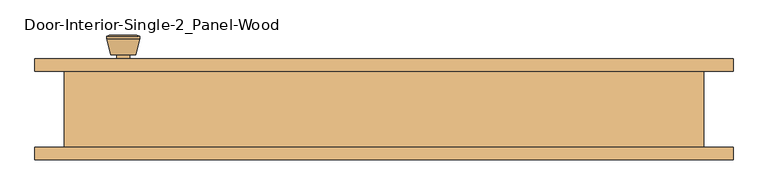
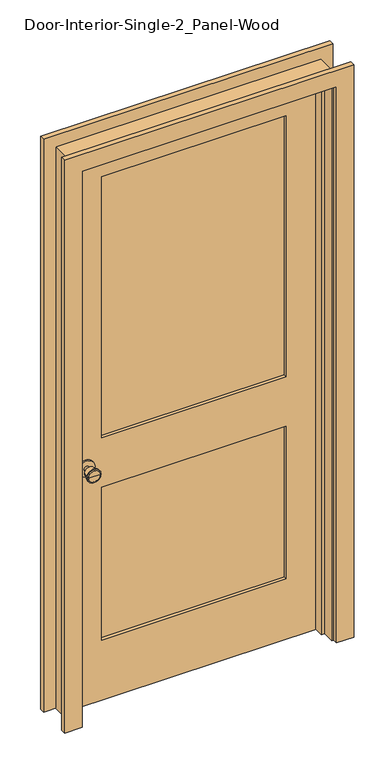
"""IFC4 building model written with IfcOpenShell, lengths in millimetres: door geometry, Door-Interior-Single-2_Panel-Wood."""

from ifc_helpers import new_model, si_unit, point, frame, frame_2d, origin, place, context, project, spatial, polyline, circle_curve, trimmed, segment, composite_curve, outline, extrude, faceted_brep, source, transform, mapped, element, save
from ifc_brep_helpers import plane_surface, cylinder_surface, revolved_surface, advanced_brep


def door_interior_single_2_panel_wood_d4071c8b(model_context):
    return source(origin(), model_context, "Body", "SolidModel", [
        advanced_brep(
        [(-393.7, 13.05, 914.4), (-383.7, 13.05, 914.4), (-403.7, 13.05, 914.4), (-373.2241324, -35.95, 914.4), (-393.7, -35.95, 914.4), (-414.1758676, -35.95, 914.4), (-368.7, -34.1221319, 914.4), (-418.7, -34.1221319, 914.4), (-368.7, -30.6584537, 914.4), (-418.7, -30.6584537, 914.4), (-375.063764, -5.95, 914.4), (-412.336236, -5.95, 914.4), (-383.7, -5.95, 914.4), (-403.7, -5.95, 914.4)],
        [
            (0, 1),
            (1, 2, circle_curve(frame((-393.7, 13.05, 914.4), z_axis=(0.0, 1.0, 0.0), x_axis=(-1.0, 0.0, 0.0)), 10.0)),
            (2, 0),
            (2, 1, circle_curve(frame((-393.7, 13.05, 914.4), z_axis=(0.0, 1.0, 0.0), x_axis=(-1.0, 0.0, 0.0)), 10.0)),
            (3, 4),
            (4, 5),
            (5, 3, circle_curve(frame((-393.7, -35.95, 914.4), z_axis=(0.0, -1.0, 0.0), x_axis=(-1.0, 0.0, 0.0)), 20.4758676)),
            (3, 5, circle_curve(frame((-393.7, -35.95, 914.4), z_axis=(0.0, -1.0, 0.0), x_axis=(-1.0, 0.0, 0.0)), 20.4758676)),
            (6, 3),
            (5, 7),
            (7, 6, circle_curve(frame((-393.7, -34.1221319, 914.4), z_axis=(0.0, -1.0, 0.0), x_axis=(-1.0, 0.0, 0.0)), 25.0)),
            (6, 7, circle_curve(frame((-393.7, -34.1221319, 914.4), z_axis=(0.0, -1.0, 0.0), x_axis=(-1.0, 0.0, 0.0)), 25.0)),
            (8, 6),
            (7, 9),
            (9, 8, circle_curve(frame((-393.7, -30.6584537, 914.4), z_axis=(0.0, -1.0, 0.0), x_axis=(-1.0, 0.0, 0.0)), 25.0)),
            (8, 9, circle_curve(frame((-393.7, -30.6584537, 914.4), z_axis=(0.0, -1.0, 0.0), x_axis=(-1.0, 0.0, 0.0)), 25.0)),
            (10, 8),
            (9, 11),
            (11, 10, circle_curve(frame((-393.7, -5.95, 914.4), z_axis=(0.0, -1.0, 0.0), x_axis=(-1.0, 0.0, 0.0)), 18.636236)),
            (10, 11, circle_curve(frame((-393.7, -5.95, 914.4), z_axis=(0.0, -1.0, 0.0), x_axis=(-1.0, 0.0, 0.0)), 18.636236)),
            (12, 10),
            (11, 13),
            (13, 12, circle_curve(frame((-393.7, -5.95, 914.4), z_axis=(0.0, -1.0, 0.0), x_axis=(-1.0, 0.0, 0.0)), 10.0)),
            (12, 13, circle_curve(frame((-393.7, -5.95, 914.4), z_axis=(0.0, -1.0, 0.0), x_axis=(-1.0, 0.0, 0.0)), 10.0)),
            (1, 12),
            (13, 2),
        ],
        [
            plane_surface(frame((-393.7, 13.05, 914.4), z_axis=(0.0, 1.0, 0.0), x_axis=(-1.0, 0.0, 0.0))),
            plane_surface(frame((-393.7, -35.95, 914.4), z_axis=(0.0, -1.0, 0.0), x_axis=(-1.0, 0.0, 0.0))),
            revolved_surface(polyline([(-414.1758676, -35.95, 914.4), (-418.7, -34.1221319, 914.4)]), (-393.7, 13.05, 914.4), (0.0, 1.0, 0.0)),
            cylinder_surface(frame((-393.7, 13.05, 914.4), z_axis=(0.0, 1.0, 0.0), x_axis=(-1.0, 0.0, 0.0)), 25.0),
            revolved_surface(polyline([(-418.7, -30.6584537, 914.4), (-412.336236, -5.95, 914.4)]), (-393.7, 13.05, 914.4), (0.0, 1.0, 0.0)),
            plane_surface(frame((-393.7, -5.95, 914.4), z_axis=(0.0, 1.0, 0.0), x_axis=(-1.0, 0.0, 0.0))),
            cylinder_surface(frame((-393.7, 13.05, 914.4), z_axis=(0.0, 1.0, 0.0), x_axis=(-1.0, 0.0, 0.0)), 10.0),
        ],
        [
            (0, [[1, 2, 3]]),
            (0, [[-3, 4, -1]]),
            (1, [[5, 6, 7]]),
            (1, [[-6, -5, 8]]),
            (2, [[9, -7, 10, 11]]),
            (2, [[-10, -8, -9, 12]]),
            (3, [[13, -11, 14, 15]]),
            (3, [[-14, -12, -13, 16]]),
            (4, [[17, -15, 18, 19]]),
            (4, [[-18, -16, -17, 20]]),
            (5, [[21, -19, 22, 23]]),
            (5, [[-22, -20, -21, 24]]),
            (6, [[25, -23, 26, -2]]),
            (6, [[-26, -24, -25, -4]]),
        ],
    ),
        extrude(outline(composite_curve([segment(trimmed(circle_curve(frame_2d((914.4, -393.7)), 30.0), [point((914.4, -423.7))], [point((914.4, -363.7))], False, "CARTESIAN"), True, "CONTINUOUS"), segment(trimmed(circle_curve(frame_2d((914.4, -393.7)), 30.0), [point((914.4, -363.7))], [point((914.4, -423.7))], False, "CARTESIAN"), True, "CONTINUOUS")], self_intersect=False)), frame((0.0, 13.05, 0.0), z_axis=(0.0, 1.0, 0.0), x_axis=(0.0, 0.0, 1.0)), (0.0, 0.0, 1.0), 6.0),
        advanced_brep(
        [(-393.7, 59.975, 914.4), (-403.7, 59.975, 914.4), (-383.7, 59.975, 914.4), (-373.2241324, 108.975, 914.4), (-414.1758676, 108.975, 914.4), (-393.7, 108.975, 914.4), (-368.7, 107.1471319, 914.4), (-418.7, 107.1471319, 914.4), (-368.7, 103.6834537, 914.4), (-418.7, 103.6834537, 914.4), (-375.063764, 78.975, 914.4), (-412.336236, 78.975, 914.4), (-383.7, 78.975, 914.4), (-403.7, 78.975, 914.4)],
        [
            (0, 1),
            (1, 2, circle_curve(frame((-393.7, 59.975, 914.4), z_axis=(0.0, -1.0, 0.0), x_axis=(-1.0, 0.0, 0.0)), 10.0)),
            (2, 0),
            (2, 1, circle_curve(frame((-393.7, 59.975, 914.4), z_axis=(0.0, -1.0, 0.0), x_axis=(-1.0, 0.0, 0.0)), 10.0)),
            (3, 4, circle_curve(frame((-393.7, 108.975, 914.4), z_axis=(0.0, 1.0, 0.0), x_axis=(-1.0, 0.0, 0.0)), 20.4758676)),
            (4, 5),
            (5, 3),
            (4, 3, circle_curve(frame((-393.7, 108.975, 914.4), z_axis=(0.0, 1.0, 0.0), x_axis=(-1.0, 0.0, 0.0)), 20.4758676)),
            (6, 7, circle_curve(frame((-393.7, 107.1471319, 914.4), z_axis=(0.0, 1.0, 0.0), x_axis=(-1.0, 0.0, 0.0)), 25.0)),
            (7, 4),
            (3, 6),
            (7, 6, circle_curve(frame((-393.7, 107.1471319, 914.4), z_axis=(0.0, 1.0, 0.0), x_axis=(-1.0, 0.0, 0.0)), 25.0)),
            (8, 9, circle_curve(frame((-393.7, 103.6834537, 914.4), z_axis=(0.0, 1.0, 0.0), x_axis=(-1.0, 0.0, 0.0)), 25.0)),
            (9, 7),
            (6, 8),
            (9, 8, circle_curve(frame((-393.7, 103.6834537, 914.4), z_axis=(0.0, 1.0, 0.0), x_axis=(-1.0, 0.0, 0.0)), 25.0)),
            (10, 11, circle_curve(frame((-393.7, 78.975, 914.4), z_axis=(0.0, 1.0, 0.0), x_axis=(-1.0, 0.0, 0.0)), 18.636236)),
            (11, 9),
            (8, 10),
            (11, 10, circle_curve(frame((-393.7, 78.975, 914.4), z_axis=(0.0, 1.0, 0.0), x_axis=(-1.0, 0.0, 0.0)), 18.636236)),
            (12, 13, circle_curve(frame((-393.7, 78.975, 914.4), z_axis=(0.0, 1.0, 0.0), x_axis=(-1.0, 0.0, 0.0)), 10.0)),
            (13, 11),
            (10, 12),
            (13, 12, circle_curve(frame((-393.7, 78.975, 914.4), z_axis=(0.0, 1.0, 0.0), x_axis=(-1.0, 0.0, 0.0)), 10.0)),
            (1, 13),
            (12, 2),
        ],
        [
            plane_surface(frame((-393.7, 59.975, 914.4), z_axis=(0.0, -1.0, 0.0), x_axis=(-1.0, 0.0, 0.0))),
            plane_surface(frame((-393.7, 108.975, 914.4), z_axis=(0.0, 1.0, 0.0), x_axis=(-1.0, 0.0, 0.0))),
            revolved_surface(polyline([(-414.1758676, 108.975, 914.4), (-418.7, 107.1471319, 914.4)]), (-393.7, 59.975, 914.4), (0.0, -1.0, 0.0)),
            cylinder_surface(frame((-393.7, 59.975, 914.4), z_axis=(0.0, -1.0, 0.0), x_axis=(-1.0, 0.0, 0.0)), 25.0),
            revolved_surface(polyline([(-418.7, 103.6834537, 914.4), (-412.336236, 78.975, 914.4)]), (-393.7, 59.975, 914.4), (0.0, -1.0, 0.0)),
            plane_surface(frame((-393.7, 78.975, 914.4), z_axis=(0.0, -1.0, 0.0), x_axis=(-1.0, 0.0, 0.0))),
            cylinder_surface(frame((-393.7, 59.975, 914.4), z_axis=(0.0, -1.0, 0.0), x_axis=(-1.0, 0.0, 0.0)), 10.0),
        ],
        [
            (0, [[1, 2, 3]]),
            (0, [[-3, 4, -1]]),
            (1, [[5, 6, 7]]),
            (1, [[8, -7, -6]]),
            (2, [[9, 10, -5, 11]]),
            (2, [[12, -11, -8, -10]]),
            (3, [[13, 14, -9, 15]]),
            (3, [[16, -15, -12, -14]]),
            (4, [[17, 18, -13, 19]]),
            (4, [[20, -19, -16, -18]]),
            (5, [[21, 22, -17, 23]]),
            (5, [[24, -23, -20, -22]]),
            (6, [[-2, 25, -21, 26]]),
            (6, [[-4, -26, -24, -25]]),
        ],
    ),
        extrude(outline(composite_curve([segment(trimmed(circle_curve(frame_2d((914.4, -393.7)), 30.0), [point((914.4, -423.7))], [point((914.4, -363.7))], False, "CARTESIAN"), True, "CONTINUOUS"), segment(trimmed(circle_curve(frame_2d((914.4, -393.7)), 30.0), [point((914.4, -363.7))], [point((914.4, -423.7))], False, "CARTESIAN"), True, "CONTINUOUS")], self_intersect=False)), frame((0.0, 53.975, 0.0), z_axis=(0.0, 1.0, 0.0), x_axis=(0.0, 0.0, 1.0)), (0.0, 0.0, 1.0), 6.0),
        faceted_brep([(482.6, 53.975, 0.0), (482.6, -60.325, 0.0), (457.2, -60.325, 0.0), (457.2, -15.875, 0.0), (444.5, -15.875, 0.0), (444.5, 19.05, 0.0), (457.2, 19.05, 0.0), (457.2, 53.975, 0.0), (482.6, 53.975, 2159.0), (482.6, -60.325, 2159.0), (-482.6, -60.325, 2159.0), (-482.6, -60.325, 0.0), (-457.2, -60.325, 0.0), (-457.2, -60.325, 2133.6), (457.2, -60.325, 2133.6), (457.2, -15.875, 2133.6), (-457.2, -15.875, 2133.6), (-457.2, -15.875, 0.0), (-444.5, -15.875, 0.0), (-444.5, -15.875, 2120.9), (444.5, -15.875, 2120.9), (444.5, 19.05, 2120.9), (-444.5, 19.05, 2120.9), (-444.5, 19.05, 0.0), (-457.2, 19.05, 0.0), (-457.2, 19.05, 2133.6), (457.2, 19.05, 2133.6), (457.2, 53.975, 2133.6), (-457.2, 53.975, 2133.6), (-457.2, 53.975, 0.0), (-482.6, 53.975, 0.0), (-482.6, 53.975, 2159.0)], [[[0, 1, 2, 3, 4, 5, 6, 7]], [[1, 0, 8, 9]], [[2, 1, 9, 10, 11, 12, 13, 14]], [[3, 2, 14, 15]], [[4, 3, 15, 16, 17, 18, 19, 20]], [[5, 4, 20, 21]], [[6, 5, 21, 22, 23, 24, 25, 26]], [[7, 6, 26, 27]], [[0, 7, 27, 28, 29, 30, 31, 8]], [[9, 8, 31, 10]], [[15, 14, 13, 16]], [[21, 20, 19, 22]], [[27, 26, 25, 28]], [[30, 29, 24, 23, 18, 17, 12, 11]], [[10, 31, 30, 11]], [[16, 13, 12, 17]], [[22, 19, 18, 23]], [[28, 25, 24, 29]]]),
        extrude(outline(polyline([(2133.6, -457.2), (0.0, -457.2), (0.0, 457.2), (2133.6, 457.2), (2133.6, -457.2)]), holes=[polyline([(2014.5375, -336.55), (2014.5375, 336.55), (1009.65, 336.55), (1009.65, -336.55), (2014.5375, -336.55)]), polyline([(819.15, -336.55), (819.15, 336.55), (231.775, 336.55), (231.775, -336.55), (819.15, -336.55)])]), frame((0.0, 19.05, 0.0), z_axis=(0.0, 1.0, 0.0), x_axis=(0.0, 0.0, 1.0)), (0.0, 0.0, 1.0), 34.925),
        extrude(outline(polyline([(336.55, 30.6916667), (-336.55, 30.6916667), (-336.55, 42.3333333), (336.55, 42.3333333), (336.55, 30.6916667)])), frame((0.0, 0.0, 1009.65), z_axis=(0.0, 0.0, 1.0), x_axis=(1.0, 0.0, 0.0)), (0.0, 0.0, 1.0), 1004.8875),
        extrude(outline(polyline([(336.55, 30.6916667), (-336.55, 30.6916667), (-336.55, 42.3333333), (336.55, 42.3333333), (336.55, 30.6916667)])), frame((0.0, 0.0, 231.775), z_axis=(0.0, 0.0, 1.0), x_axis=(1.0, 0.0, 0.0)), (0.0, 0.0, 1.0), 587.375),
        extrude(outline(polyline([(0.0, 463.55), (0.0, 527.05), (2203.45, 527.05), (2203.45, -527.05), (0.0, -527.05), (0.0, -463.55), (2139.95, -463.55), (2139.95, 463.55), (0.0, 463.55)])), frame((0.0, 53.975, 0.0), z_axis=(0.0, 1.0, 0.0), x_axis=(0.0, 0.0, 1.0)), (0.0, 0.0, 1.0), 19.05),
        extrude(outline(polyline([(0.0, 463.55), (0.0, 527.05), (2203.45, 527.05), (2203.45, -527.05), (0.0, -527.05), (0.0, -463.55), (2139.95, -463.55), (2139.95, 463.55), (0.0, 463.55)])), frame((0.0, -79.375, 0.0), z_axis=(0.0, 1.0, 0.0), x_axis=(0.0, 0.0, 1.0)), (0.0, 0.0, 1.0), 19.05),
    ])


if __name__ == "__main__":
    model = new_model("IFC4")
    model_context = context("Model", 3, world=origin())
    ifc_project = project(units=[si_unit("LENGTHUNIT", "METRE", prefix="MILLI")], contexts=[model_context])
    site = spatial("IfcSite", under=ifc_project)
    building = spatial("IfcBuilding", under=site)
    placement = place(None, origin())
    door_interior_single_2_panel_wood_shape = door_interior_single_2_panel_wood_d4071c8b(model_context)
    element("IfcDoor", 1, ObjectType="Door-Interior-Single-2_Panel-Wood", at=placement, inside=building, context=model_context, shape_type="MappedRepresentation", body=[
        mapped(door_interior_single_2_panel_wood_shape, transform((0.0, 0.0, 0.0), x_axis=(1.0, 0.0, 0.0), y_axis=(0.0, 1.0, 0.0), z_axis=(0.0, 0.0, 1.0))),
    ])
    save(model, "model.ifc")

# Revit data of these elements
# Type "Door-Interior-Single-2_Panel-Wood"
#   Type Mark = "10"
#   Assembly Code = "C1020300"
#   Analytic Construction = "Wooden"
#   Top Rail = 0' - 4 11/16"
#   Thickness = 0' - 1 3/8"
#   Thermal Resistance (R) = 2.5876 (h·ft²·°F)/BTU
#   Swing Angle [instance default] = 90.00°
#   Stiles = 0' - 4 3/4"
#   Rough Width = 3' - 2"
#   Rough Height = 7' - 1"
#   Lock Rail = 0' - 7 1/2"
#   Height = 7' - 0"
#   Width = 3' - 0"
#   Heat Transfer Coefficient (U) = 0.3865 BTU/(h·ft²·°F)
#   Bottom Rail = 0' - 9 1/8"
#   Trim Material = Cherry
#   Panel Material = Cherry
#   Frame Material = Cherry
#   Door Handle Material = Aluminum
#   Visual Light Transmittance = 0
#   Solar Heat Gain Coefficient = 0
#   Wall Closure = (empty or 0)
#   Function = (empty or 0)
# Element 1 (IfcDoor, "Door-Interior-Single-2_Panel-Wood")
#   Materials on its faces: "Cherry", "Aluminum"
# Materials
#   "Cherry": class "Wood", colour RGB 226 177 128, transparency 0, Description = "Prunus Serotina", Cost = 0
#   "Aluminum": class "Metal", colour RGB 247 247 247, transparency 0, Description = "Aluminum 6061", Cost = 0
